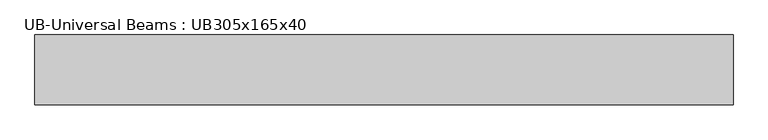
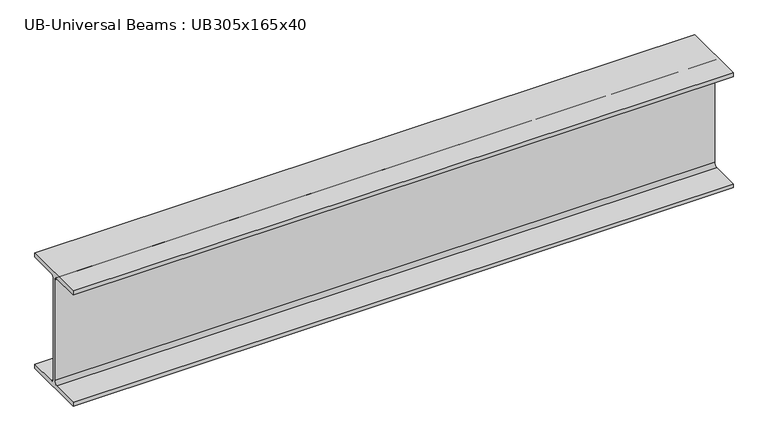
"""IFC4 building model written with IfcOpenShell, lengths in millimetres: beam geometry, UB-Universal Beams : UB305x165x40."""

from ifc_helpers import new_model, si_unit, point, frame, frame_2d, origin, place, context, project, spatial, polyline, circle_curve, trimmed, segment, composite_curve, outline, extrude, source, transform, mapped, element, save


def ub_universal_beams_ub305x165x40_8a566974(model_context):
    return source(origin(), model_context, "Body", "SweptSolid", [
        extrude(outline(composite_curve([segment(polyline([(82.5, -141.5), (82.5, -151.7), (-82.5, -151.7), (-82.5, -141.5), (-11.9, -141.5)]), True, "CONTINUOUS"), segment(trimmed(circle_curve(frame_2d((-11.9, -132.6)), 8.9), [point((-11.9, -141.5))], [point((-3.0, -132.6))], True, "CARTESIAN"), True, "CONTINUOUS"), segment(polyline([(-3.0, -132.6), (-3.0, 132.6)]), True, "CONTINUOUS"), segment(trimmed(circle_curve(frame_2d((-11.9, 132.6)), 8.9), [point((-3.0, 132.6))], [point((-11.9, 141.5))], True, "CARTESIAN"), True, "CONTINUOUS"), segment(polyline([(-11.9, 141.5), (-82.5, 141.5), (-82.5, 151.7), (82.5, 151.7), (82.5, 141.5), (11.9, 141.5)]), True, "CONTINUOUS"), segment(trimmed(circle_curve(frame_2d((11.9, 132.6)), 8.9), [point((11.9, 141.5))], [point((3.0, 132.6))], True, "CARTESIAN"), True, "CONTINUOUS"), segment(polyline([(3.0, 132.6), (3.0, -132.6)]), True, "CONTINUOUS"), segment(trimmed(circle_curve(frame_2d((11.9, -132.6)), 8.9), [point((3.0, -132.6))], [point((11.9, -141.5))], True, "CARTESIAN"), True, "CONTINUOUS"), segment(polyline([(11.9, -141.5), (82.5, -141.5)]), True, "CONTINUOUS")], self_intersect=False)), frame((-835.6, 0.0, 0.0), z_axis=(1.0, 0.0, 0.0), x_axis=(0.0, 1.0, 0.0)), (0.0, 0.0, 1.0), 1645.4),
    ])


if __name__ == "__main__":
    model = new_model("IFC4")
    model_context = context("Model", 3, world=origin())
    ifc_project = project(units=[si_unit("LENGTHUNIT", "METRE", prefix="MILLI")], contexts=[model_context])
    site = spatial("IfcSite", under=ifc_project)
    building = spatial("IfcBuilding", under=site)
    placement = place(None, origin())
    ub_universal_beams_ub305x165x40_shape = ub_universal_beams_ub305x165x40_8a566974(model_context)
    element("IfcBeam", 1, ObjectType="UB-Universal Beams : UB305x165x40", at=placement, inside=building, context=model_context, shape_type="MappedRepresentation", body=[
        mapped(ub_universal_beams_ub305x165x40_shape, transform((0.0, 0.0, 0.0), x_axis=(1.0, 0.0, 0.0), y_axis=(0.0, 1.0, 0.0), z_axis=(0.0, 0.0, 1.0))),
    ])
    save(model, "model.ifc")

# Revit data of these elements
# Type "UB-Universal Beams : UB305x165x40"
#   Section Name Key = "UB305X165X40"
#   Width = 16.5 cm
#   Web Thickness = 0.6 cm
#   Web Fillet = 0.89 cm
#   Warping Constant = 164000.0 cm⁶
#   Torsional Moment of Inertia = 14.70 cm⁴
#   Section Area = 51.3 cm²
#   Plastic Modulus weak axis = 142.0 cm³
#   Plastic Modulus strong axis = 623.0 cm³
#   Nominal Weight = 40.2999 kgf/m
#   Moment of Inertia weak axis = 764.00 cm⁴
#   Moment of Inertia strong axis = 8503.00 cm⁴
#   Height = 30.34 cm
#   Flange Thickness = 1.02 cm
#   Elastic Modulus weak axis = 92.6 cm³
#   Elastic Modulus strong axis = 560.0 cm³
#   Centroid Vertical = 15.17 cm
#   Centroid Horizontal = 8.25 cm
#   Bolt Spacing = 9.0 cm
#   Length [instance default] = 1500 mm
#   Structural Material [instance default] = Metal - Steel 43-275
#   Type Comments = ""
#   Assembly Code = ""
# Element 1 (IfcBeam, "UB-Universal Beams : UB305x165x40")
#   Materials on its faces: "Metal - Steel 43-275"
# Materials
#   "Metal - Steel 43-275": class "Metal", colour RGB 247 247 247, transparency 0, Cost = 0
